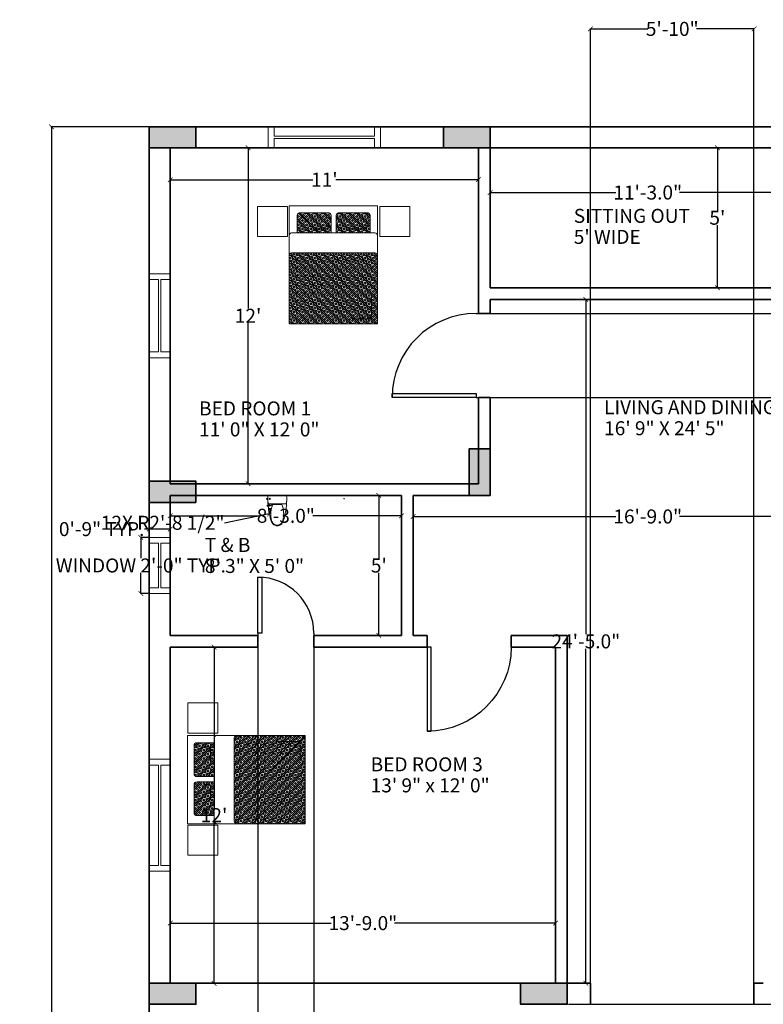
# Model space of a CAD drawing. Units: inches. Extents: x 560 to 1118, y 291 to 1226.
# Tile 3 of 4: x 560 to 878, y 804 to 1226. Entities that reach past the tile are written whole.
import ezdxf

# ---------------------------------------------------------------- set-up
doc = ezdxf.new("R2010")
doc.units = ezdxf.units.IN
doc.header["$MEASUREMENT"] = 0
for name, color, linetype, lineweight in [('A-ANNO-DIMS', 2, 'Continuous', 13), ('A-AREA-IDEN', 7, 'Continuous', 18), ('A-COLS', 7, 'Continuous', 35), ('A-FLOR-FIXT', 9, 'Continuous', 18), ('DOORS', 4, 'Continuous', 25), ('FURNITURE', 8, 'Continuous', 18), ('WALL', 7, 'Continuous', 35), ('WINDOWS', 80, 'Continuous', 18)]:
    doc.layers.add(name, color=color, linetype=linetype, lineweight=lineweight)
doc.styles.get("Standard").update_dxf_attribs({"font": 'arial.ttf'})
doc.dimstyles.get("Standard").update_dxf_attribs({"dimtxt": 6, "dimasz": 2, "dimexe": 0.18, "dimexo": 0.0625, "dimgap": 0.09, "dimtad": 0, "dimtih": 1, "dimtoh": 1, "dimdec": 1, "dimzin": 0, "dimdsep": 46, "dimlunit": 3, "dimtxsty": 'Standard', "dimblk": 'ARCHTICK', "dimcen": 0.09, "dimadec": 0, "dimazin": 0, "dimtfac": 1, "dimtdec": 1, "dimtofl": 0, "dimtmove": 0, "dimatfit": 3, "dimfxl": 1, "dimtolj": 1, "dimtzin": 0, "dimarcsym": 0})
pattern_1 = [(135, (-1377.70473, -125.71507), (-0.070710678, -0.070710678), []), (135, (-1377.68705, -125.69739), (-0.070710678, -0.070710678), []), (45, (-1377.70473, -125.71507), (-0.070710678, 0.070710678), [-0.025, 0.025]), (45, (-1377.72241, -125.69739), (-0.070710678, 0.070710678), [-0.025, 0.025]), (45, (-1377.74009, -125.67972), (-0.070710678, 0.070710678), [0.025, -0.025]), (45, (-1377.75776, -125.66204), (-0.070710678, 0.070710678), [0.025, -0.025]), (135, (-1377.66938, -125.67972), (-0.070710678, -0.070710678), [0.025, -0.025]), (135, (-1377.6517, -125.66204), (-0.070710678, -0.070710678), [0.025, -0.025])]

# ---------------------------------------------------------------- blocks, each defined once
blk = doc.blocks.new('*U3')
for p, q in [((0, 0), (0, -6)), ((36, 0), (36, -6))]:
    blk.add_line(p, q)
blk.add_lwpolyline([(0, 0), (0, 36), (1.75, 36), (1.75, 0)], close=True)
blk.add_arc((0, 0), 36, 0, 90)
blk = doc.blocks.new('*U5')
for p, q in [((0, 0), (0, -5)), ((36, 0), (36, -5))]:
    blk.add_line(p, q)
blk.add_lwpolyline([(0, 0), (0, 36), (1.75, 36), (1.75, 0)], close=True)
blk.add_arc((0, 0), 36, 0, 90)
blk = doc.blocks.new('*U4')
for p, q in [((0, 0), (0, -6)), ((24, 0), (24, -6))]:
    blk.add_line(p, q)
blk.add_lwpolyline([(0, 0), (0, 24), (1.75, 24), (1.75, 0)], close=True)
blk.add_arc((0, 0), 24, 0, 90)
blk = doc.blocks.new('_ArchTick')
at = {"color": 0, "linetype": 'ByBlock', "const_width": 0.15}
blk.add_lwpolyline([(-0.5, -0.5), (0.5, 0.5)], dxfattribs=at)
blk = doc.blocks.new('*D6')
at = {"layer": 'A-ANNO-DIMS', "color": 0, "lineweight": -2, "transparency": 16777216}
for p, q in [((657.5, 1171), (657.5, 1102.1)), ((657.56, 1171), (657.68, 1171)), ((657.5, 1027), (657.5, 1095.9)), ((657.56, 1027), (657.68, 1027))]:
    blk.add_line(p, q, dxfattribs=at)
at = {"layer": 'Defpoints', "color": 0, "transparency": 16777216}
for p in [(657.5, 1171), (657.5, 1027), (657.5, 1027)]:
    blk.add_point(p, dxfattribs=at)
at = {"layer": 'A-ANNO-DIMS', "color": 0, "lineweight": -2, "transparency": 16777216, "xscale": 2, "yscale": 2, "zscale": 2}
for p, rotation in [((657.5, 1171), 90), ((657.5, 1027), 270)]:
    blk.add_blockref('_ArchTick', p, dxfattribs=dict(at, rotation=rotation))
at = {"layer": 'A-ANNO-DIMS', "color": 0, "transparency": 16777216, "insert": (657.5, 1099), "char_height": 6, "attachment_point": 5}
blk.add_mtext("\\A1;12'", dxfattribs=at)
blk = doc.blocks.new('*D7')
at = {"layer": 'A-ANNO-DIMS', "color": 0, "lineweight": -2, "transparency": 16777216}
for p, q in [((624.18, 1157.74), (624.18, 1157.12)), ((624.18, 1157.3), (685.28, 1157.3)), ((756.18, 1157.3), (695.08, 1157.3)), ((756.18, 1157.74), (756.18, 1157.12))]:
    blk.add_line(p, q, dxfattribs=at)
at = {"layer": 'Defpoints', "color": 0, "transparency": 16777216}
for p in [(624.18, 1157.8), (756.18, 1157.8), (756.18, 1157.3)]:
    blk.add_point(p, dxfattribs=at)
at = {"layer": 'A-ANNO-DIMS', "color": 0, "lineweight": -2, "transparency": 16777216, "xscale": 2, "yscale": 2, "zscale": 2, "rotation": 180}
blk.add_blockref('_ArchTick', (624.18, 1157.3), dxfattribs=at)
at = {"layer": 'A-ANNO-DIMS', "color": 0, "lineweight": -2, "transparency": 16777216, "xscale": 2, "yscale": 2, "zscale": 2}
blk.add_blockref('_ArchTick', (756.18, 1157.3), dxfattribs=at)
at = {"layer": 'A-ANNO-DIMS', "color": 0, "transparency": 16777216, "insert": (690.18, 1157.3), "char_height": 6, "attachment_point": 5}
blk.add_mtext("\\A1;11'", dxfattribs=at)
blk = doc.blocks.new('*D8')
at = {"layer": 'A-ANNO-DIMS', "color": 0, "lineweight": -2, "transparency": 16777216}
for p, q in [((761.18, 1149.36), (761.18, 1151.98)), ((761.18, 1151.8), (815.07, 1151.8)), ((896.18, 1151.8), (842.29, 1151.8)), ((896.18, 1149.36), (896.18, 1151.98))]:
    blk.add_line(p, q, dxfattribs=at)
at = {"layer": 'Defpoints', "color": 0, "transparency": 16777216}
for p in [(896.18, 1151.8), (761.18, 1149.3), (896.18, 1149.3)]:
    blk.add_point(p, dxfattribs=at)
at = {"layer": 'A-ANNO-DIMS', "color": 0, "lineweight": -2, "transparency": 16777216, "xscale": 2, "yscale": 2, "zscale": 2, "rotation": 180}
blk.add_blockref('_ArchTick', (761.18, 1151.8), dxfattribs=at)
at = {"layer": 'A-ANNO-DIMS', "color": 0, "lineweight": -2, "transparency": 16777216, "xscale": 2, "yscale": 2, "zscale": 2}
blk.add_blockref('_ArchTick', (896.18, 1151.8), dxfattribs=at)
at = {"layer": 'A-ANNO-DIMS', "color": 0, "transparency": 16777216, "insert": (828.68, 1151.8), "char_height": 6, "attachment_point": 5}
blk.add_mtext('\\A1;11\'-3.0"', dxfattribs=at)
blk = doc.blocks.new('*D9')
at = {"layer": 'A-ANNO-DIMS', "color": 0, "lineweight": -2, "transparency": 16777216}
for p, q in [((854.56, 1171), (858.68, 1171)), ((858.5, 1171), (858.5, 1144.14)), ((858.5, 1111), (858.5, 1137.86)), ((854.56, 1111), (858.68, 1111))]:
    blk.add_line(p, q, dxfattribs=at)
at = {"layer": 'Defpoints', "color": 0, "transparency": 16777216}
for p in [(854.5, 1171), (854.5, 1111), (858.5, 1111)]:
    blk.add_point(p, dxfattribs=at)
at = {"layer": 'A-ANNO-DIMS', "color": 0, "lineweight": -2, "transparency": 16777216, "xscale": 2, "yscale": 2, "zscale": 2}
for p, rotation in [((858.5, 1171), 90), ((858.5, 1111), 270)]:
    blk.add_blockref('_ArchTick', p, dxfattribs=dict(at, rotation=rotation))
at = {"layer": 'A-ANNO-DIMS', "color": 0, "transparency": 16777216, "insert": (858.5, 1141), "char_height": 6, "attachment_point": 5}
blk.add_mtext("\\A1;5'", dxfattribs=at)
blk = doc.blocks.new('*D12')
at = {"layer": 'A-ANNO-DIMS', "color": 0, "lineweight": -2, "transparency": 16777216}
for p, q in [((713.94, 1022), (713.32, 1022)), ((713.5, 1022), (713.5, 995.14)), ((713.5, 962), (713.5, 988.86)), ((713.94, 962), (713.32, 962))]:
    blk.add_line(p, q, dxfattribs=at)
at = {"layer": 'Defpoints', "color": 0, "transparency": 16777216}
for p in [(714, 1022), (713.5, 962), (714, 962)]:
    blk.add_point(p, dxfattribs=at)
at = {"layer": 'A-ANNO-DIMS', "color": 0, "lineweight": -2, "transparency": 16777216, "xscale": 2, "yscale": 2, "zscale": 2}
for p, rotation in [((713.5, 1022), 90), ((713.5, 962), 270)]:
    blk.add_blockref('_ArchTick', p, dxfattribs=dict(at, rotation=rotation))
at = {"layer": 'A-ANNO-DIMS', "color": 0, "transparency": 16777216, "insert": (713.5, 992), "char_height": 6, "attachment_point": 5}
blk.add_mtext("\\A1;5'", dxfattribs=at)
blk = doc.blocks.new('*D13')
at = {"layer": 'A-ANNO-DIMS', "color": 0, "lineweight": -2, "transparency": 16777216}
for p, q in [((624.18, 1013.36), (624.18, 1013.48)), ((624.18, 1013.3), (662.12, 1013.3)), ((723.18, 1013.3), (685.24, 1013.3)), ((723.18, 1013.36), (723.18, 1013.48))]:
    blk.add_line(p, q, dxfattribs=at)
at = {"layer": 'Defpoints', "color": 0, "transparency": 16777216}
for p in [(624.18, 1013.3), (723.18, 1013.3), (723.18, 1013.3)]:
    blk.add_point(p, dxfattribs=at)
at = {"layer": 'A-ANNO-DIMS', "color": 0, "lineweight": -2, "transparency": 16777216, "xscale": 2, "yscale": 2, "zscale": 2, "rotation": 180}
blk.add_blockref('_ArchTick', (624.18, 1013.3), dxfattribs=at)
at = {"layer": 'A-ANNO-DIMS', "color": 0, "lineweight": -2, "transparency": 16777216, "xscale": 2, "yscale": 2, "zscale": 2}
blk.add_blockref('_ArchTick', (723.18, 1013.3), dxfattribs=at)
at = {"layer": 'A-ANNO-DIMS', "color": 0, "transparency": 16777216, "insert": (673.68, 1013.3), "char_height": 6, "attachment_point": 5}
blk.add_mtext('\\A1;8\'-3.0"', dxfattribs=at)
blk = doc.blocks.new('*D32')
at = {"layer": 'A-ANNO-DIMS', "color": 0, "lineweight": -2, "transparency": 16777216}
for p, q in [((642.93, 957), (642.93, 888.1)), ((642.99, 957), (643.11, 957)), ((642.93, 813), (642.93, 881.9)), ((642.99, 813), (643.11, 813))]:
    blk.add_line(p, q, dxfattribs=at)
at = {"layer": 'Defpoints', "color": 0, "transparency": 16777216}
for p in [(642.93, 957), (642.93, 813), (642.93, 813)]:
    blk.add_point(p, dxfattribs=at)
at = {"layer": 'A-ANNO-DIMS', "color": 0, "lineweight": -2, "transparency": 16777216, "xscale": 2, "yscale": 2, "zscale": 2}
for p, rotation in [((642.93, 957), 90), ((642.93, 813), 270)]:
    blk.add_blockref('_ArchTick', p, dxfattribs=dict(at, rotation=rotation))
at = {"layer": 'A-ANNO-DIMS', "color": 0, "transparency": 16777216, "insert": (642.93, 885), "char_height": 6, "attachment_point": 5}
blk.add_mtext("\\A1;12'", dxfattribs=at)
blk = doc.blocks.new('*D33')
at = {"layer": 'A-ANNO-DIMS', "color": 0, "lineweight": -2, "transparency": 16777216}
for p, q in [((624.18, 838.86), (624.18, 838.98)), ((624.18, 838.8), (693.07, 838.8)), ((789.18, 838.8), (720.29, 838.8)), ((789.18, 838.86), (789.18, 838.98))]:
    blk.add_line(p, q, dxfattribs=at)
at = {"layer": 'Defpoints', "color": 0, "transparency": 16777216}
for p in [(624.18, 838.8), (789.18, 838.8), (789.18, 838.8)]:
    blk.add_point(p, dxfattribs=at)
at = {"layer": 'A-ANNO-DIMS', "color": 0, "lineweight": -2, "transparency": 16777216, "xscale": 2, "yscale": 2, "zscale": 2, "rotation": 180}
blk.add_blockref('_ArchTick', (624.18, 838.8), dxfattribs=at)
at = {"layer": 'A-ANNO-DIMS', "color": 0, "lineweight": -2, "transparency": 16777216, "xscale": 2, "yscale": 2, "zscale": 2}
blk.add_blockref('_ArchTick', (789.18, 838.8), dxfattribs=at)
at = {"layer": 'A-ANNO-DIMS', "color": 0, "transparency": 16777216, "insert": (706.68, 838.8), "char_height": 6, "attachment_point": 5}
blk.add_mtext('\\A1;13\'-9.0"', dxfattribs=at)
blk = doc.blocks.new('*D38')
at = {"layer": 'A-ANNO-DIMS', "color": 0, "lineweight": -2, "transparency": 16777216}
for p, q in [((796.56, 1106), (802.36, 1106)), ((802.18, 1106), (802.18, 962.65)), ((802.18, 813), (802.18, 956.35)), ((796.56, 813), (802.36, 813))]:
    blk.add_line(p, q, dxfattribs=at)
at = {"layer": 'Defpoints', "color": 0, "transparency": 16777216}
for p in [(796.5, 1106), (796.5, 813), (802.18, 813)]:
    blk.add_point(p, dxfattribs=at)
at = {"layer": 'A-ANNO-DIMS', "color": 0, "lineweight": -2, "transparency": 16777216, "xscale": 2, "yscale": 2, "zscale": 2}
for p, rotation in [((802.18, 1106), 90), ((802.18, 813), 270)]:
    blk.add_blockref('_ArchTick', p, dxfattribs=dict(at, rotation=rotation))
at = {"layer": 'A-ANNO-DIMS', "color": 0, "transparency": 16777216, "insert": (802.18, 959.5), "char_height": 6, "attachment_point": 5}
blk.add_mtext('\\A1;24\'-5.0"', dxfattribs=at)
blk = doc.blocks.new('*D39')
at = {"layer": 'A-ANNO-DIMS', "color": 0, "lineweight": -2, "transparency": 16777216}
for p, q in [((728.18, 1015.74), (728.18, 1012.82)), ((728.18, 1013), (815.07, 1013)), ((929.18, 1013), (842.29, 1013)), ((929.18, 1015.74), (929.18, 1012.82))]:
    blk.add_line(p, q, dxfattribs=at)
at = {"layer": 'Defpoints', "color": 0, "transparency": 16777216}
for p in [(728.18, 1015.8), (929.18, 1015.8), (929.18, 1013)]:
    blk.add_point(p, dxfattribs=at)
at = {"layer": 'A-ANNO-DIMS', "color": 0, "lineweight": -2, "transparency": 16777216, "xscale": 2, "yscale": 2, "zscale": 2, "rotation": 180}
blk.add_blockref('_ArchTick', (728.18, 1013), dxfattribs=at)
at = {"layer": 'A-ANNO-DIMS', "color": 0, "lineweight": -2, "transparency": 16777216, "xscale": 2, "yscale": 2, "zscale": 2}
blk.add_blockref('_ArchTick', (929.18, 1013), dxfattribs=at)
at = {"layer": 'A-ANNO-DIMS', "color": 0, "transparency": 16777216, "insert": (828.68, 1013), "char_height": 6, "attachment_point": 5}
blk.add_mtext('\\A1;16\'-9.0"', dxfattribs=at)
blk = doc.blocks.new('MAT-P10')
h = blk.add_hatch()
h.set_pattern_fill('BOX', color=256, scale=0.1, angle=45, style=0)
h.set_pattern_definition(pattern_1)
h.paths.add_polyline_path([(-0.157, 1.46), (0.417, 1.46), (0.417, 1.751, 0.414214), (0.367, 1.801), (-0.107, 1.801, 0.414214), (-0.157, 1.751)])
h.paths.add_polyline_path([(0.505, 1.46), (1.079, 1.46), (1.079, 1.751, 0.414214), (1.029, 1.801), (0.555, 1.801, 0.414214), (0.505, 1.751)])
h = blk.add_hatch()
h.set_pattern_fill('BOX', color=256, scale=0.1, angle=45, style=0)
h.set_pattern_definition(pattern_1)
edge = h.paths.add_edge_path()
edge.add_line((1.205, -0.085), (1.205, 1.062))
edge.add_ellipse((1.161, 1.063), major_axis=(0, 0.0568), ratio=0.776379, start_angle=270, end_angle=360)
edge.add_line((1.161, 1.119), (-0.251, 1.12))
edge.add_ellipse((-0.251, 1.063), major_axis=(0, 0.0568), ratio=0.776379, start_angle=0, end_angle=88.1396)
edge.add_line((-0.295, 1.064), (-0.295, -0.085))
edge.add_line((-0.295, -0.085), (1.205, -0.085))
for p, q in [((-0.251, 1.46), (1.161, 1.46)), ((-0.251, 1.12), (1.161, 1.119)), ((1.102, 0.406), (1.102, 0.057)), ((1.058, 0), (0.775, 0))]:
    blk.add_line(p, q)
for points in [[(-0.83, 1.909), (-0.319, 1.909), (-0.319, 1.398), (-0.83, 1.398)], [(1.205, -0.085), (-0.295, -0.085), (-0.295, 1.915), (1.205, 1.915)], [(1.244, 1.909), (1.755, 1.909), (1.755, 1.398), (1.244, 1.398)]]:
    blk.add_lwpolyline(points, close=True)
for points in [[(0.417, 1.46), (0.417, 1.751, 0.414214), (0.367, 1.801), (-0.107, 1.801, 0.414214), (-0.157, 1.751), (-0.157, 1.46)], [(1.079, 1.46), (1.079, 1.751, 0.414214), (1.029, 1.801), (0.555, 1.801, 0.414214), (0.505, 1.751), (0.505, 1.46)], [(0.37, 1.624), (0.37, 1.571, -0.414214), (0.32, 1.521), (0.111, 1.521)], [(1.012, 1.644), (1.012, 1.571, -0.414214), (0.962, 1.521), (0.753, 1.521)]]:
    blk.add_lwpolyline(points, format="xyb")
at = {"extrusion": (0, 0, -1)}
for centre, start_param, end_param in [((-0.251, 1.404), 4.712389, 6.283185), ((1.161, 1.404), 0, 1.570796), ((-0.251, 1.063), 4.712389, 6.283185), ((1.161, 1.063), 0, 1.570796), ((1.058, 0.057), 1.570796, 3.141593), ((1.058, 0.057), 1.570796, 3.141593)]:
    blk.add_ellipse(centre, major_axis=(0, 0.0568), ratio=0.776379, start_param=start_param, end_param=end_param, dxfattribs=at)
blk = doc.blocks.new('toilet-7')
at = {"color": 0, "linetype": 'ByBlock'}
for p, q in [((-0.246, -0.087), (-0.246, -0.107)), ((-0.246, -0.087), (-0.226, -0.087)), ((-0.246, -0.107), (-0.226, -0.107)), ((-0.226, -0.085), (-0.226, -0.11)), ((-0.226, -0.085), (-0.216, -0.085)), ((-0.226, -0.11), (-0.215, -0.11)), ((0.21, -0.02), (-0.21, -0.02)), ((0.199, -0.212), (-0.199, -0.212)), ((-0.18, -0.237), (-0.18, -0.212)), ((-0.121, -0.237), (-0.121, -0.212)), ((-0.102, -0.221), (0.102, -0.221)), ((0.199, -0.212), (0.21, -0.164)), ((0.215, -0.068), (0.21, -0.02)), ((0.21, -0.164), (0.215, -0.117)), ((0.215, -0.117), (0.215, -0.068)), ((-0.121, -0.237), (-0.228, -0.237)), ((-0.228, -0.237), (-0.228, -0.26)), ((-0.176, -0.26), (-0.228, -0.26)), ((-0.176, -0.26), (-0.138, -0.245)), ((-0.138, -0.245), (-0.138, -0.237))]:
    blk.add_line(p, q, dxfattribs=at)
blk.add_circle((-0.17, -0.097), 0.0125, dxfattribs=at)
for centre, radius, start, end in [((0.224, -0.092), 0.44, 170.5377, 187.7399), ((1.517, -0.087), 1.732, 181.2224, 184.9822), ((0.224, -0.092), 0.44, 187.7399, 195.822), ((0.426, -0.441), 0.572, 157.3737, 194.7786), ((-0.426, -0.441), 0.572, 345.2214, 22.6263), ((-1.517, -0.087), 1.732, 342.7523, 358.7776), ((1.517, -0.087), 1.732, 185.7323, 197.2477), ((0.012, -0.554), 0.155, 197.2477, 249.5476), ((0.022, -0.548), 0.155, 194.7786, 226.8543), ((0, -0.571), 0.122, 226.8543, 313.1457), ((-0.012, -0.554), 0.155, 290.4524, 342.7523), ((-0.022, -0.548), 0.155, 313.1457, 345.2214), ((0, -0.585), 0.122, 249.5476, 290.4524)]:
    blk.add_arc(centre, radius, start, end, dxfattribs=at)
blk = doc.blocks.new('WIN-48IN')
for p, q in [((0, 9), (48, 9)), ((0, 0), (0, 9)), ((2.5, 5), (2.5, 9)), ((45.5, 9), (45.5, 5)), ((48, 9), (48, 0)), ((2.5, 5), (45.5, 5)), ((48, 0), (0, 0)), ((2.5, 0), (2.5, 4)), ((2.5, 4), (45.5, 4)), ((45.5, 4), (45.5, 0))]:
    blk.add_line(p, q)
blk = doc.blocks.new('WIN-36IN')
for p, q in [((0, 0), (0, 36)), ((0, 36), (9, 36)), ((9, 36), (9, 0)), ((0, 33.5), (4, 33.5)), ((4, 33.5), (4, 2.5)), ((5, 33.5), (9, 33.5)), ((5, 33.5), (5, 2.5)), ((4, 2.5), (0, 2.5)), ((9, 0), (0, 0)), ((9, 2.5), (5, 2.5))]:
    blk.add_line(p, q)
blk = doc.blocks.new('WIN-24IN')
for p, q in [((0, 0), (0, 24)), ((0, 24), (9, 24)), ((0, 21.5), (4, 21.5)), ((4, 21.5), (4, 2.5)), ((5, 21.5), (9, 21.5)), ((5, 21.5), (5, 2.5)), ((9, 24), (9, 0)), ((4, 2.5), (0, 2.5)), ((9, 0), (0, 0)), ((9, 2.5), (5, 2.5))]:
    blk.add_line(p, q)
blk = doc.blocks.new('COL-RECT-9X20-NOM')
h = blk.add_hatch(color=256)
h.dxf.hatch_style = 1
h.paths.add_polyline_path([(19.98, 0), (19.98, 9), (0, 9), (0, 0)])
blk.add_lwpolyline([(0, 9), (0, 0), (19.98, 0), (19.98, 9)], close=True)
blk = doc.blocks.new('*D67')
at = {"layer": 'A-ANNO-DIMS', "color": 0, "lineweight": -2, "transparency": 16777216}
for p, q in [((615.12, 1004), (611.4, 1004)), ((611.58, 1004), (611.58, 995.19)), ((611.58, 980), (611.58, 988.81)), ((615.12, 980), (611.4, 980))]:
    blk.add_line(p, q, dxfattribs=at)
at = {"layer": 'Defpoints', "color": 0, "transparency": 16777216}
for p in [(615.18, 1004), (611.58, 980), (615.18, 980)]:
    blk.add_point(p, dxfattribs=at)
at = {"layer": 'A-ANNO-DIMS', "color": 0, "lineweight": -2, "transparency": 16777216, "xscale": 2, "yscale": 2, "zscale": 2}
for p, rotation in [((611.58, 1004), 90), ((611.58, 980), 270)]:
    blk.add_blockref('_ArchTick', p, dxfattribs=dict(at, rotation=rotation))
at = {"layer": 'A-ANNO-DIMS', "color": 0, "transparency": 16777216, "insert": (611.58, 992), "char_height": 6, "attachment_point": 5}
blk.add_mtext('\\A1;WINDOW 2\'-0" TYP.', dxfattribs=at)
blk = doc.blocks.new('*D68')
at = {"layer": 'A-ANNO-DIMS', "color": 0, "lineweight": -2, "transparency": 16777216}
for p, q in [((615.18, 1007.6), (613.18, 1007.6)), ((615.18, 1004.06), (615.18, 1007.78)), ((624.18, 1007.6), (615.18, 1007.6)), ((624.18, 1004.06), (624.18, 1007.78))]:
    blk.add_line(p, q, dxfattribs=at)
at = {"layer": 'Defpoints', "color": 0, "transparency": 16777216}
for p in [(615.18, 1007.6), (615.18, 1004), (624.18, 1004)]:
    blk.add_point(p, dxfattribs=at)
at = {"layer": 'A-ANNO-DIMS', "color": 0, "lineweight": -2, "transparency": 16777216, "xscale": 2, "yscale": 2, "zscale": 2, "rotation": 180}
blk.add_blockref('_ArchTick', (615.18, 1007.6), dxfattribs=at)
at = {"layer": 'A-ANNO-DIMS', "color": 0, "lineweight": -2, "transparency": 16777216, "xscale": 2, "yscale": 2, "zscale": 2}
blk.add_blockref('_ArchTick', (624.18, 1007.6), dxfattribs=at)
at = {"layer": 'A-ANNO-DIMS', "color": 0, "transparency": 16777216, "insert": (594.8, 1007.6), "char_height": 6, "attachment_point": 5}
blk.add_mtext('\\A1;0\'-9" TYP.', dxfattribs=at)
blk = doc.blocks.new('*D72')
at = {"layer": 'A-ANNO-DIMS', "color": 0, "lineweight": -2, "transparency": 16777216}
for p, q in [((615.12, 1180), (573.1, 1180)), ((573.28, 1180), (573.28, 764.15)), ((573.28, 342), (573.28, 757.85)), ((615.12, 342), (573.1, 342))]:
    blk.add_line(p, q, dxfattribs=at)
at = {"layer": 'Defpoints', "color": 0, "transparency": 16777216}
for p in [(573.28, 1180), (615.18, 1180), (615.18, 342)]:
    blk.add_point(p, dxfattribs=at)
at = {"layer": 'A-ANNO-DIMS', "color": 0, "lineweight": -2, "transparency": 16777216, "xscale": 2, "yscale": 2, "zscale": 2}
for p, rotation in [((573.28, 1180), 90), ((573.28, 342), 270)]:
    blk.add_blockref('_ArchTick', p, dxfattribs=dict(at, rotation=rotation))
at = {"layer": 'A-ANNO-DIMS', "color": 0, "transparency": 16777216, "insert": (573.28, 761), "char_height": 6, "attachment_point": 5}
blk.add_mtext('\\A1;69\'-10"', dxfattribs=at)
blk = doc.blocks.new('*D73')
at = {"layer": 'A-ANNO-DIMS', "color": 0, "lineweight": -2, "transparency": 16777216}
for p, q in [((756.24, 1100), (1084.26, 1100)), ((1084.08, 1100), (1084.08, 1085.16)), ((1084.08, 1064), (1084.08, 1078.84)), ((756.24, 1064), (1084.26, 1064))]:
    blk.add_line(p, q, dxfattribs=at)
at = {"layer": 'Defpoints', "color": 0, "transparency": 16777216}
for p in [(756.18, 1100), (1084.08, 1100), (756.18, 1064)]:
    blk.add_point(p, dxfattribs=at)
at = {"layer": 'A-ANNO-DIMS', "color": 0, "lineweight": -2, "transparency": 16777216, "xscale": 2, "yscale": 2, "zscale": 2}
for p, rotation in [((1084.08, 1100), 90), ((1084.08, 1064), 270)]:
    blk.add_blockref('_ArchTick', p, dxfattribs=dict(at, rotation=rotation))
at = {"layer": 'A-ANNO-DIMS', "color": 0, "transparency": 16777216, "insert": (1084.08, 1082), "char_height": 6, "attachment_point": 5}
blk.add_mtext('\\A1;3\'-0"', dxfattribs=at)
blk = doc.blocks.new('*D74')
at = {"layer": 'A-ANNO-DIMS', "color": 0, "lineweight": -2, "transparency": 16777216}
for p, q in [((661.68, 961.94), (661.68, 299.92)), ((685.68, 961.94), (685.68, 299.92)), ((661.68, 300.1), (665.56, 300.1)), ((685.68, 300.1), (681.8, 300.1))]:
    blk.add_line(p, q, dxfattribs=at)
at = {"layer": 'Defpoints', "color": 0, "transparency": 16777216}
for p in [(661.68, 962), (685.68, 962), (685.68, 300.1)]:
    blk.add_point(p, dxfattribs=at)
at = {"layer": 'A-ANNO-DIMS', "color": 0, "lineweight": -2, "transparency": 16777216, "xscale": 2, "yscale": 2, "zscale": 2, "rotation": 180}
blk.add_blockref('_ArchTick', (661.68, 300.1), dxfattribs=at)
at = {"layer": 'A-ANNO-DIMS', "color": 0, "lineweight": -2, "transparency": 16777216, "xscale": 2, "yscale": 2, "zscale": 2}
blk.add_blockref('_ArchTick', (685.68, 300.1), dxfattribs=at)
at = {"layer": 'A-ANNO-DIMS', "color": 0, "transparency": 16777216, "insert": (673.68, 300.1), "char_height": 6, "attachment_point": 5}
blk.add_mtext('\\A1;2\'-0"', dxfattribs=at)
blk = doc.blocks.new('*D75')
at = {"layer": 'A-ANNO-DIMS', "color": 0, "lineweight": -2, "transparency": 16777216}
for p, q in [((804.18, 804.06), (804.18, 1222.08)), ((804.18, 1221.9), (828.78, 1221.9)), ((874.18, 1221.9), (849.58, 1221.9)), ((874.18, 804.06), (874.18, 1222.08))]:
    blk.add_line(p, q, dxfattribs=at)
at = {"layer": 'Defpoints', "color": 0, "transparency": 16777216}
for p in [(874.18, 1221.9), (804.18, 804), (874.18, 804)]:
    blk.add_point(p, dxfattribs=at)
at = {"layer": 'A-ANNO-DIMS', "color": 0, "lineweight": -2, "transparency": 16777216, "xscale": 2, "yscale": 2, "zscale": 2, "rotation": 180}
blk.add_blockref('_ArchTick', (804.18, 1221.9), dxfattribs=at)
at = {"layer": 'A-ANNO-DIMS', "color": 0, "lineweight": -2, "transparency": 16777216, "xscale": 2, "yscale": 2, "zscale": 2}
blk.add_blockref('_ArchTick', (874.18, 1221.9), dxfattribs=at)
at = {"layer": 'A-ANNO-DIMS', "color": 0, "transparency": 16777216, "insert": (839.18, 1221.9), "char_height": 6, "attachment_point": 5}
blk.add_mtext('\\A1;5\'-10"', dxfattribs=at)
blk = doc.blocks.new('*D78')
at = {"layer": 'A-ANNO-DIMS', "color": 0, "lineweight": -2, "transparency": 16777216}
for p, q in [((794.7, 804), (1084.26, 804)), ((1084.08, 804), (1084.08, 789.16)), ((1084.08, 768), (1084.08, 782.84)), ((794.7, 768), (1084.26, 768))]:
    blk.add_line(p, q, dxfattribs=at)
at = {"layer": 'Defpoints', "color": 0, "transparency": 16777216}
for p in [(794.64, 804), (1084.08, 804), (794.64, 768)]:
    blk.add_point(p, dxfattribs=at)
at = {"layer": 'A-ANNO-DIMS', "color": 0, "lineweight": -2, "transparency": 16777216, "xscale": 2, "yscale": 2, "zscale": 2}
for p, rotation in [((1084.08, 804), 90), ((1084.08, 768), 270)]:
    blk.add_blockref('_ArchTick', p, dxfattribs=dict(at, rotation=rotation))
at = {"layer": 'A-ANNO-DIMS', "color": 0, "transparency": 16777216, "insert": (1084.08, 786), "char_height": 6, "attachment_point": 5}
blk.add_mtext('\\A1;3\'-0"', dxfattribs=at)
blk = doc.blocks.new('*D80')
at = {"layer": 'A-ANNO-DIMS', "color": 0, "lineweight": -2, "transparency": 16777216}
for p, q in [((698.59, 1020.73), (698.77, 1020.73)), ((698.68, 1020.64), (698.68, 1020.82)), ((647.35, 1010.3), (666.6, 1014.21))]:
    blk.add_line(p, q, dxfattribs=at)
at = {"layer": 'Defpoints', "color": 0, "transparency": 16777216}
for p in [(698.68, 1020.73), (666.6, 1014.21)]:
    blk.add_point(p, dxfattribs=at)
at = {"layer": 'A-ANNO-DIMS', "color": 0, "lineweight": -2, "transparency": 16777216, "xscale": 2, "yscale": 2, "zscale": 2, "rotation": 11.48949137086492}
blk.add_blockref('_ArchTick', (666.6, 1014.21), dxfattribs=at)
at = {"layer": 'A-ANNO-DIMS', "color": 0, "transparency": 16777216, "insert": (620.93, 1010.3), "char_height": 6, "attachment_point": 5}
blk.add_mtext('\\A1;12X R2\'-8 1/2"', dxfattribs=at)

msp = doc.modelspace()

# ---------------------------------------------------------------- linework, layer by layer
at = {"layer": 'WALL'}
for p, q in [((615.18, 1180), (615.18, 342)), ((761.18, 1180), (615.18, 1180)), ((761.18, 1180), (761.18, 1111)), ((761.18, 1180), (896.18, 1180)), ((624.18, 1171), (624.18, 1027)), ((756.18, 1171), (624.18, 1171)), ((756.18, 1171), (756.18, 1100)), ((761.18, 1171), (896.18, 1171)), ((896.18, 1111), (761.18, 1111)), ((896.18, 1106), (761.18, 1106)), ((761.18, 1106), (761.18, 1100)), ((761.18, 1100), (756.18, 1100)), ((761.18, 1064), (756.18, 1064)), ((756.18, 1064), (756.18, 1027)), ((761.18, 1064), (761.18, 1022)), ((752.18, 1027), (624.18, 1027)), ((756.18, 1027), (752.18, 1027)), ((624.18, 1022), (624.18, 962)), ((723.18, 1022), (624.18, 1022)), ((723.18, 1022), (723.18, 962)), ((728.18, 1022), (728.18, 962)), ((752.18, 1022), (728.18, 1022)), ((761.18, 1022), (752.18, 1022)), ((661.68, 962), (624.18, 962)), ((661.68, 962), (661.68, 957)), ((723.18, 962), (685.68, 962)), ((685.68, 962), (685.68, 957)), ((734.18, 962), (728.18, 962)), ((734.18, 962), (734.18, 957)), ((794.18, 962), (770.18, 962)), ((770.18, 962), (770.18, 957)), ((794.18, 962), (794.18, 813)), ((624.18, 957), (624.18, 813)), ((661.68, 957), (624.18, 957)), ((734.18, 957), (685.68, 957)), ((789.18, 957), (770.18, 957)), ((789.18, 957), (789.18, 813)), ((789.18, 813), (624.18, 813)), ((789.18, 813), (761.18, 813)), ((800.18, 813), (794.18, 813)), ((800.18, 813), (794.18, 813)), ((800.18, 813), (804.18, 813)), ((804.18, 813), (804.18, 804)), ((874.18, 804), (874.18, 813)), ((874.18, 813), (878.18, 813))]:
    msp.add_line(p, q, dxfattribs=at)

# ---------------------------------------------------------------- block references
at = {"layer": 'A-COLS'}
for p in [(615.18, 1171), (741.2, 1171), (615.18, 804), (774.2, 804)]:
    msp.add_blockref('COL-RECT-9X20-NOM', p, dxfattribs=at)
for p, rotation in [((752.18, 1041.98), 270.0000000000001), ((635.16, 1028.06), 180)]:
    msp.add_blockref('COL-RECT-9X20-NOM', p, dxfattribs=dict(at, rotation=rotation))
at = {"layer": 'A-FLOR-FIXT', "xscale": 18.9039470471375, "yscale": 18.9039470471375, "zscale": 18.9039470471375}
msp.add_blockref('toilet-7', (670, 1022.38), dxfattribs=at)
at = {"layer": 'DOORS', "rotation": 90}
msp.add_blockref('*U3', (755.18, 1064), dxfattribs=at)
at = {"layer": 'DOORS'}
msp.add_blockref('*U4', (661.68, 963), dxfattribs=at)
at = {"layer": 'DOORS', "xscale": -1, "rotation": 180}
msp.add_blockref('*U5', (734.18, 957), dxfattribs=at)
at = {"layer": 'FURNITURE', "xscale": 25.25, "yscale": 25.25, "zscale": 25.25}
msp.add_blockref('MAT-P10', (682.51, 1097.67), dxfattribs=at)
at = {"layer": 'FURNITURE', "xscale": 25.25, "yscale": 25.25, "zscale": 25.25, "rotation": 90}
msp.add_blockref('MAT-P10', (679.86, 888.81), dxfattribs=at)
at = {"layer": 'WINDOWS'}
for name, p in [('WIN-48IN', (666.18, 1171)), ('WIN-36IN', (615.18, 1081))]:
    msp.add_blockref(name, p, dxfattribs=at)
for name, p, rotation in [('WIN-24IN', (624.18, 1004), 180), ('WIN-48IN', (615.18, 909), 270.0000000000002)]:
    msp.add_blockref(name, p, dxfattribs=dict(at, rotation=rotation))

# ---------------------------------------------------------------- texts
at = {"layer": 'A-AREA-IDEN'}
for s, p in [('SITTING OUT', (797, 1138.8)), ("5' WIDE", (797, 1129.8)), ('BED ROOM 1', (636.5, 1056.3)), ('LIVING AND DINING', (810, 1056.8)), ('11\' 0" X 12\' 0"', (636.5, 1047.3)), ('16\' 9" X 24\' 5"', (810, 1047.8)), ('T & B', (639, 997.8)), ('8\' 3" X 5\' 0"', (639, 988.8)), ('BED ROOM 3 ', (710, 903.8)), ('13\' 9" x 12\' 0"', (710, 894.8))]:
    msp.add_text(s, height=6, dxfattribs=at).set_placement(p)

# ---------------------------------------------------------------- dimensions: what is measured, and where the dimension line sits
at = {"layer": 'A-ANNO-DIMS'}
for base, p1, p2, override, picture, middle in [((874.18, 1221.9), (804.18, 804), (874.18, 804), {"dimdec": 1, "dimlfac": 1, "dimrnd": 0, "dimzin": 1, "dimdsep": 46, "dimlunit": 4, "dimfrac": 2}, '*D75', (839.18, 1221.9)), ((756.18, 1157.3), (624.18, 1157.8), (756.18, 1157.8), {"dimclrd": 0, "dimclre": 0, "dimclrt": 0}, '*D7', (690.18, 1157.3)), ((896.18, 1151.8), (761.18, 1149.3), (896.18, 1149.3), {"dimclrd": 0, "dimclre": 0, "dimclrt": 0}, '*D8', (828.68, 1151.8)), ((723.18, 1013.3), (624.18, 1013.3), (723.18, 1013.3), {"dimclrd": 0, "dimclre": 0, "dimclrt": 0}, '*D13', (673.68, 1013.3)), ((929.18, 1013), (728.18, 1015.8), (929.18, 1015.8), {"dimclrd": 0, "dimclre": 0, "dimclrt": 0}, '*D39', (828.68, 1013)), ((685.68, 300.1), (661.68, 962), (685.68, 962), {"dimdec": 1, "dimlfac": 1, "dimrnd": 0, "dimzin": 1, "dimdsep": 46, "dimlunit": 4, "dimfrac": 2}, '*D74', (673.68, 300.1)), ((789.18, 838.8), (624.18, 838.8), (789.18, 838.8), {"dimclrd": 0, "dimclre": 0, "dimclrt": 0}, '*D33', (706.68, 838.8))]:
    dim = msp.add_linear_dim(base=base, p1=p1, p2=p2, dimstyle='Standard', override=override, dxfattribs=at)
    dim.commit()
    dim.dimension.update_dxf_attribs({"geometry": picture, "text_midpoint": middle})
for base, p1, p2, override, picture, middle in [((573.28, 1180), (615.18, 342), (615.18, 1180), {"dimdec": 1, "dimlfac": 1, "dimrnd": 0, "dimzin": 1, "dimdsep": 46, "dimlunit": 4, "dimfrac": 2}, '*D72', (573.28, 761)), ((657.5, 1027), (657.5, 1171), (657.5, 1027), {"dimclrd": 0, "dimclre": 0, "dimclrt": 0}, '*D6', (657.5, 1099)), ((858.5, 1111), (854.5, 1171), (854.5, 1111), {"dimclrd": 0, "dimclre": 0, "dimclrt": 0}, '*D9', (858.5, 1141)), ((802.18, 813), (796.5, 1106), (796.5, 813), {"dimclrd": 0, "dimclre": 0, "dimclrt": 0}, '*D38', (802.18, 959.5)), ((1084.08, 1100), (756.18, 1064), (756.18, 1100), {"dimdec": 1, "dimlfac": 1, "dimrnd": 0, "dimzin": 1, "dimdsep": 46, "dimlunit": 4, "dimfrac": 2}, '*D73', (1084.08, 1082)), ((713.5, 962), (714, 1022), (714, 962), {"dimclrd": 0, "dimclre": 0, "dimclrt": 0}, '*D12', (713.5, 992)), ((642.93, 813), (642.93, 957), (642.93, 813), {"dimclrd": 0, "dimclre": 0, "dimclrt": 0}, '*D32', (642.93, 885)), ((1084.08, 804), (794.64, 768), (794.64, 804), {"dimdec": 1, "dimlfac": 1, "dimrnd": 0, "dimzin": 1, "dimdsep": 46, "dimlunit": 4, "dimfrac": 2}, '*D78', (1084.08, 786))]:
    dim = msp.add_linear_dim(base=base, p1=p1, p2=p2, angle=90, dimstyle='Standard', override=override, dxfattribs=at)
    dim.commit()
    dim.dimension.update_dxf_attribs({"geometry": picture, "text_midpoint": middle})
dim = msp.add_radius_dim(center=(698.68, 1020.73), mpoint=(666.6, 1014.21), text='12X <>', dimstyle='Standard', override={"dimdec": 1, "dimlfac": 1, "dimrnd": 0, "dimzin": 1, "dimdsep": 46, "dimlunit": 4, "dimfrac": 2}, dxfattribs=at)
dim.commit()
dim.dimension.update_dxf_attribs({"geometry": '*D80', "text_midpoint": (647.35, 1010.3), "dimtype": 164})
for base, p1, p2, angle, text, picture, middle in [((615.18, 1007.6), (624.18, 1004), (615.18, 1004), 180, '<> TYP.', '*D68', (594.8, 1007.6)), ((611.58, 980), (615.18, 1004), (615.18, 980), 270, 'WINDOW <> TYP.', '*D67', (611.58, 992))]:
    dim = msp.add_linear_dim(base=base, p1=p1, p2=p2, angle=angle, text=text, dimstyle='Standard', override={"dimdec": 1, "dimlfac": 1, "dimrnd": 0, "dimzin": 1, "dimdsep": 46, "dimlunit": 4, "dimfrac": 2}, dxfattribs=at)
    dim.commit()
    dim.dimension.update_dxf_attribs({"geometry": picture, "text_midpoint": middle})

doc.saveas('drawing.dxf')
